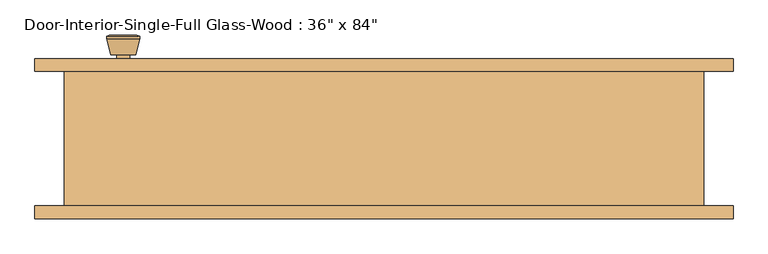
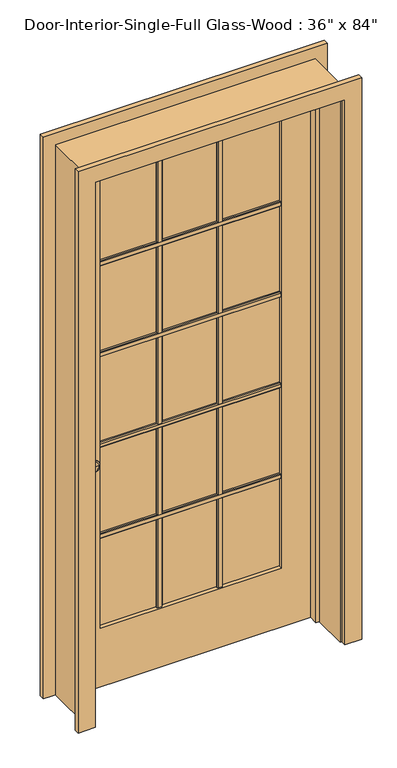
"""IFC4 building model written with IfcOpenShell, lengths in millimetres: door geometry."""

from ifc_helpers import new_model, si_unit, point, frame, frame_2d, origin, place, context, project, spatial, polyline, circle_curve, trimmed, segment, composite_curve, outline, extrude, faceted_brep, source, transform, mapped, element, save
from ifc_brep_helpers import plane_surface, cylinder_surface, revolved_surface, advanced_brep


def door_cfd81529(model_context):
    return source(origin(), model_context, "Body", "SolidModel", [
        extrude(outline(polyline([(84.455, 1667.51), (90.805, 1667.51), (93.98, 1664.335), (93.98, 1651.635), (90.805, 1648.46), (84.455, 1648.46), (84.455, 1667.51)])), frame((-336.55, 0.0, 0.0), z_axis=(1.0, 0.0, 0.0), x_axis=(0.0, 1.0, 0.0)), (0.0, 0.0, 1.0), 673.1),
        extrude(outline(polyline([(84.455, 1310.9575), (90.805, 1310.9575), (93.98, 1307.7825), (93.98, 1295.0825), (90.805, 1291.9075), (84.455, 1291.9075), (84.455, 1310.9575)])), frame((-336.55, 0.0, 0.0), z_axis=(1.0, 0.0, 0.0), x_axis=(0.0, 1.0, 0.0)), (0.0, 0.0, 1.0), 673.1),
        extrude(outline(polyline([(84.455, 954.405), (90.805, 954.405), (93.98, 951.23), (93.98, 938.53), (90.805, 935.355), (84.455, 935.355), (84.455, 954.405)])), frame((-336.55, 0.0, 0.0), z_axis=(1.0, 0.0, 0.0), x_axis=(0.0, 1.0, 0.0)), (0.0, 0.0, 1.0), 673.1),
        extrude(outline(polyline([(84.455, 597.8525), (90.805, 597.8525), (93.98, 594.6775), (93.98, 581.9775), (90.805, 578.8025), (84.455, 578.8025), (84.455, 597.8525)])), frame((-336.55, 0.0, 0.0), z_axis=(1.0, 0.0, 0.0), x_axis=(0.0, 1.0, 0.0)), (0.0, 0.0, 1.0), 673.1),
        extrude(outline(polyline([(102.6583333, 84.455), (102.6583333, 90.805), (105.8333333, 93.98), (118.5333333, 93.98), (121.7083333, 90.805), (121.7083333, 84.455), (102.6583333, 84.455)])), frame((0.0, 0.0, 231.775), z_axis=(0.0, 0.0, 1.0), x_axis=(1.0, 0.0, 0.0)), (0.0, 0.0, 1.0), 1782.7625),
        extrude(outline(polyline([(-121.7083333, 84.455), (-121.7083333, 90.805), (-118.5333333, 93.98), (-105.8333333, 93.98), (-102.6583333, 90.805), (-102.6583333, 84.455), (-121.7083333, 84.455)])), frame((0.0, 0.0, 231.775), z_axis=(0.0, 0.0, 1.0), x_axis=(1.0, 0.0, 0.0)), (0.0, 0.0, 1.0), 1782.7625),
        extrude(outline(polyline([(77.47, 1667.51), (77.47, 1648.46), (71.12, 1648.46), (67.945, 1651.635), (67.945, 1664.335), (71.12, 1667.51), (77.47, 1667.51)])), frame((-336.55, 0.0, 0.0), z_axis=(1.0, 0.0, 0.0), x_axis=(0.0, 1.0, 0.0)), (0.0, 0.0, 1.0), 673.1),
        extrude(outline(polyline([(77.47, 1310.9575), (77.47, 1291.9075), (71.12, 1291.9075), (67.945, 1295.0825), (67.945, 1307.7825), (71.12, 1310.9575), (77.47, 1310.9575)])), frame((-336.55, 0.0, 0.0), z_axis=(1.0, 0.0, 0.0), x_axis=(0.0, 1.0, 0.0)), (0.0, 0.0, 1.0), 673.1),
        extrude(outline(polyline([(77.47, 954.405), (77.47, 935.355), (71.12, 935.355), (67.945, 938.53), (67.945, 951.23), (71.12, 954.405), (77.47, 954.405)])), frame((-336.55, 0.0, 0.0), z_axis=(1.0, 0.0, 0.0), x_axis=(0.0, 1.0, 0.0)), (0.0, 0.0, 1.0), 673.1),
        extrude(outline(polyline([(77.47, 597.8525), (77.47, 578.8025), (71.12, 578.8025), (67.945, 581.9775), (67.945, 594.6775), (71.12, 597.8525), (77.47, 597.8525)])), frame((-336.55, 0.0, 0.0), z_axis=(1.0, 0.0, 0.0), x_axis=(0.0, 1.0, 0.0)), (0.0, 0.0, 1.0), 673.1),
        extrude(outline(polyline([(102.6583333, 77.47), (121.7083333, 77.47), (121.7083333, 71.12), (118.5333333, 67.945), (105.8333333, 67.945), (102.6583333, 71.12), (102.6583333, 77.47)])), frame((0.0, 0.0, 231.775), z_axis=(0.0, 0.0, 1.0), x_axis=(1.0, 0.0, 0.0)), (0.0, 0.0, 1.0), 1782.7625),
        extrude(outline(polyline([(-121.7083333, 77.47), (-102.6583333, 77.47), (-102.6583333, 71.12), (-105.8333333, 67.945), (-118.5333333, 67.945), (-121.7083333, 71.12), (-121.7083333, 77.47)])), frame((0.0, 0.0, 231.775), z_axis=(0.0, 0.0, 1.0), x_axis=(1.0, 0.0, 0.0)), (0.0, 0.0, 1.0), 1782.7625),
        advanced_brep(
        [(-393.7, 57.5, 914.4), (-383.7, 57.5, 914.4), (-403.7, 57.5, 914.4), (-373.2241324, 8.5, 914.4), (-393.7, 8.5, 914.4), (-414.1758676, 8.5, 914.4), (-368.7, 10.3278681, 914.4), (-418.7, 10.3278681, 914.4), (-368.7, 13.7915463, 914.4), (-418.7, 13.7915463, 914.4), (-375.063764, 38.5, 914.4), (-412.336236, 38.5, 914.4), (-383.7, 38.5, 914.4), (-403.7, 38.5, 914.4)],
        [
            (0, 1),
            (1, 2, circle_curve(frame((-393.7, 57.5, 914.4), z_axis=(0.0, 1.0, 0.0), x_axis=(-1.0, 0.0, 0.0)), 10.0)),
            (2, 0),
            (2, 1, circle_curve(frame((-393.7, 57.5, 914.4), z_axis=(0.0, 1.0, 0.0), x_axis=(-1.0, 0.0, 0.0)), 10.0)),
            (3, 4),
            (4, 5),
            (5, 3, circle_curve(frame((-393.7, 8.5, 914.4), z_axis=(0.0, -1.0, 0.0), x_axis=(-1.0, 0.0, 0.0)), 20.4758676)),
            (3, 5, circle_curve(frame((-393.7, 8.5, 914.4), z_axis=(0.0, -1.0, 0.0), x_axis=(-1.0, 0.0, 0.0)), 20.4758676)),
            (6, 3),
            (5, 7),
            (7, 6, circle_curve(frame((-393.7, 10.3278681, 914.4), z_axis=(0.0, -1.0, 0.0), x_axis=(-1.0, 0.0, 0.0)), 25.0)),
            (6, 7, circle_curve(frame((-393.7, 10.3278681, 914.4), z_axis=(0.0, -1.0, 0.0), x_axis=(-1.0, 0.0, 0.0)), 25.0)),
            (8, 6),
            (7, 9),
            (9, 8, circle_curve(frame((-393.7, 13.7915463, 914.4), z_axis=(0.0, -1.0, 0.0), x_axis=(-1.0, 0.0, 0.0)), 25.0)),
            (8, 9, circle_curve(frame((-393.7, 13.7915463, 914.4), z_axis=(0.0, -1.0, 0.0), x_axis=(-1.0, 0.0, 0.0)), 25.0)),
            (10, 8),
            (9, 11),
            (11, 10, circle_curve(frame((-393.7, 38.5, 914.4), z_axis=(0.0, -1.0, 0.0), x_axis=(-1.0, 0.0, 0.0)), 18.636236)),
            (10, 11, circle_curve(frame((-393.7, 38.5, 914.4), z_axis=(0.0, -1.0, 0.0), x_axis=(-1.0, 0.0, 0.0)), 18.636236)),
            (12, 10),
            (11, 13),
            (13, 12, circle_curve(frame((-393.7, 38.5, 914.4), z_axis=(0.0, -1.0, 0.0), x_axis=(-1.0, 0.0, 0.0)), 10.0)),
            (12, 13, circle_curve(frame((-393.7, 38.5, 914.4), z_axis=(0.0, -1.0, 0.0), x_axis=(-1.0, 0.0, 0.0)), 10.0)),
            (1, 12),
            (13, 2),
        ],
        [
            plane_surface(frame((-393.7, 57.5, 914.4), z_axis=(0.0, 1.0, 0.0), x_axis=(-1.0, 0.0, 0.0))),
            plane_surface(frame((-393.7, 8.5, 914.4), z_axis=(0.0, -1.0, 0.0), x_axis=(-1.0, 0.0, 0.0))),
            revolved_surface(polyline([(-414.1758676, 8.5, 914.4), (-418.7, 10.3278681, 914.4)]), (-393.7, 57.5, 914.4), (0.0, 1.0, 0.0)),
            cylinder_surface(frame((-393.7, 57.5, 914.4), z_axis=(0.0, 1.0, 0.0), x_axis=(-1.0, 0.0, 0.0)), 25.0),
            revolved_surface(polyline([(-418.7, 13.7915463, 914.4), (-412.336236, 38.5, 914.4)]), (-393.7, 57.5, 914.4), (0.0, 1.0, 0.0)),
            plane_surface(frame((-393.7, 38.5, 914.4), z_axis=(0.0, 1.0, 0.0), x_axis=(-1.0, 0.0, 0.0))),
            cylinder_surface(frame((-393.7, 57.5, 914.4), z_axis=(0.0, 1.0, 0.0), x_axis=(-1.0, 0.0, 0.0)), 10.0),
        ],
        [
            (0, [[1, 2, 3]]),
            (0, [[-3, 4, -1]]),
            (1, [[5, 6, 7]]),
            (1, [[-6, -5, 8]]),
            (2, [[9, -7, 10, 11]]),
            (2, [[-10, -8, -9, 12]]),
            (3, [[13, -11, 14, 15]]),
            (3, [[-14, -12, -13, 16]]),
            (4, [[17, -15, 18, 19]]),
            (4, [[-18, -16, -17, 20]]),
            (5, [[21, -19, 22, 23]]),
            (5, [[-22, -20, -21, 24]]),
            (6, [[25, -23, 26, -2]]),
            (6, [[-26, -24, -25, -4]]),
        ],
    ),
        extrude(outline(composite_curve([segment(trimmed(circle_curve(frame_2d((914.4, -393.7)), 30.0), [point((914.4, -423.7))], [point((914.4, -363.7))], False, "CARTESIAN"), True, "CONTINUOUS"), segment(trimmed(circle_curve(frame_2d((914.4, -393.7)), 30.0), [point((914.4, -363.7))], [point((914.4, -423.7))], False, "CARTESIAN"), True, "CONTINUOUS")], self_intersect=False)), frame((0.0, 57.5, 0.0), z_axis=(0.0, 1.0, 0.0), x_axis=(0.0, 0.0, 1.0)), (0.0, 0.0, 1.0), 6.0),
        advanced_brep(
        [(-393.7, 104.425, 914.4), (-403.7, 104.425, 914.4), (-383.7, 104.425, 914.4), (-373.2241324, 153.425, 914.4), (-414.1758676, 153.425, 914.4), (-393.7, 153.425, 914.4), (-368.7, 151.5971319, 914.4), (-418.7, 151.5971319, 914.4), (-368.7, 148.1334537, 914.4), (-418.7, 148.1334537, 914.4), (-375.063764, 123.425, 914.4), (-412.336236, 123.425, 914.4), (-383.7, 123.425, 914.4), (-403.7, 123.425, 914.4)],
        [
            (0, 1),
            (1, 2, circle_curve(frame((-393.7, 104.425, 914.4), z_axis=(0.0, -1.0, 0.0), x_axis=(-1.0, 0.0, 0.0)), 10.0)),
            (2, 0),
            (2, 1, circle_curve(frame((-393.7, 104.425, 914.4), z_axis=(0.0, -1.0, 0.0), x_axis=(-1.0, 0.0, 0.0)), 10.0)),
            (3, 4, circle_curve(frame((-393.7, 153.425, 914.4), z_axis=(0.0, 1.0, 0.0), x_axis=(-1.0, 0.0, 0.0)), 20.4758676)),
            (4, 5),
            (5, 3),
            (4, 3, circle_curve(frame((-393.7, 153.425, 914.4), z_axis=(0.0, 1.0, 0.0), x_axis=(-1.0, 0.0, 0.0)), 20.4758676)),
            (6, 7, circle_curve(frame((-393.7, 151.5971319, 914.4), z_axis=(0.0, 1.0, 0.0), x_axis=(-1.0, 0.0, 0.0)), 25.0)),
            (7, 4),
            (3, 6),
            (7, 6, circle_curve(frame((-393.7, 151.5971319, 914.4), z_axis=(0.0, 1.0, 0.0), x_axis=(-1.0, 0.0, 0.0)), 25.0)),
            (8, 9, circle_curve(frame((-393.7, 148.1334537, 914.4), z_axis=(0.0, 1.0, 0.0), x_axis=(-1.0, 0.0, 0.0)), 25.0)),
            (9, 7),
            (6, 8),
            (9, 8, circle_curve(frame((-393.7, 148.1334537, 914.4), z_axis=(0.0, 1.0, 0.0), x_axis=(-1.0, 0.0, 0.0)), 25.0)),
            (10, 11, circle_curve(frame((-393.7, 123.425, 914.4), z_axis=(0.0, 1.0, 0.0), x_axis=(-1.0, 0.0, 0.0)), 18.636236)),
            (11, 9),
            (8, 10),
            (11, 10, circle_curve(frame((-393.7, 123.425, 914.4), z_axis=(0.0, 1.0, 0.0), x_axis=(-1.0, 0.0, 0.0)), 18.636236)),
            (12, 13, circle_curve(frame((-393.7, 123.425, 914.4), z_axis=(0.0, 1.0, 0.0), x_axis=(-1.0, 0.0, 0.0)), 10.0)),
            (13, 11),
            (10, 12),
            (13, 12, circle_curve(frame((-393.7, 123.425, 914.4), z_axis=(0.0, 1.0, 0.0), x_axis=(-1.0, 0.0, 0.0)), 10.0)),
            (1, 13),
            (12, 2),
        ],
        [
            plane_surface(frame((-393.7, 104.425, 914.4), z_axis=(0.0, -1.0, 0.0), x_axis=(-1.0, 0.0, 0.0))),
            plane_surface(frame((-393.7, 153.425, 914.4), z_axis=(0.0, 1.0, 0.0), x_axis=(-1.0, 0.0, 0.0))),
            revolved_surface(polyline([(-414.1758676, 153.425, 914.4), (-418.7, 151.5971319, 914.4)]), (-393.7, 104.425, 914.4), (0.0, -1.0, 0.0)),
            cylinder_surface(frame((-393.7, 104.425, 914.4), z_axis=(0.0, -1.0, 0.0), x_axis=(-1.0, 0.0, 0.0)), 25.0),
            revolved_surface(polyline([(-418.7, 148.1334537, 914.4), (-412.336236, 123.425, 914.4)]), (-393.7, 104.425, 914.4), (0.0, -1.0, 0.0)),
            plane_surface(frame((-393.7, 123.425, 914.4), z_axis=(0.0, -1.0, 0.0), x_axis=(-1.0, 0.0, 0.0))),
            cylinder_surface(frame((-393.7, 104.425, 914.4), z_axis=(0.0, -1.0, 0.0), x_axis=(-1.0, 0.0, 0.0)), 10.0),
        ],
        [
            (0, [[1, 2, 3]]),
            (0, [[-3, 4, -1]]),
            (1, [[5, 6, 7]]),
            (1, [[8, -7, -6]]),
            (2, [[9, 10, -5, 11]]),
            (2, [[12, -11, -8, -10]]),
            (3, [[13, 14, -9, 15]]),
            (3, [[16, -15, -12, -14]]),
            (4, [[17, 18, -13, 19]]),
            (4, [[20, -19, -16, -18]]),
            (5, [[21, 22, -17, 23]]),
            (5, [[24, -23, -20, -22]]),
            (6, [[-2, 25, -21, 26]]),
            (6, [[-4, -26, -24, -25]]),
        ],
    ),
        extrude(outline(composite_curve([segment(trimmed(circle_curve(frame_2d((914.4, -393.7)), 30.0), [point((914.4, -423.7))], [point((914.4, -363.7))], False, "CARTESIAN"), True, "CONTINUOUS"), segment(trimmed(circle_curve(frame_2d((914.4, -393.7)), 30.0), [point((914.4, -363.7))], [point((914.4, -423.7))], False, "CARTESIAN"), True, "CONTINUOUS")], self_intersect=False)), frame((0.0, 98.425, 0.0), z_axis=(0.0, 1.0, 0.0), x_axis=(0.0, 0.0, 1.0)), (0.0, 0.0, 1.0), 6.0),
        extrude(outline(polyline([(2133.6, -457.2), (0.0, -457.2), (0.0, 457.2), (2133.6, 457.2), (2133.6, -457.2)]), holes=[polyline([(2014.5375, -336.55), (2014.5375, 336.55), (231.775, 336.55), (231.775, -336.55), (2014.5375, -336.55)])]), frame((0.0, 63.5, 0.0), z_axis=(0.0, 1.0, 0.0), x_axis=(0.0, 0.0, 1.0)), (0.0, 0.0, 1.0), 34.925),
        faceted_brep([(482.6, 98.425, 0.0), (482.6, -104.775, 0.0), (457.2, -104.775, 0.0), (457.2, 28.575, 0.0), (444.5, 28.575, 0.0), (444.5, 63.5, 0.0), (457.2, 63.5, 0.0), (457.2, 98.425, 0.0), (482.6, 98.425, 2159.0), (482.6, -104.775, 2159.0), (-482.6, -104.775, 2159.0), (-482.6, -104.775, 0.0), (-457.2, -104.775, 0.0), (-457.2, -104.775, 2133.6), (457.2, -104.775, 2133.6), (457.2, 28.575, 2133.6), (-457.2, 28.575, 2133.6), (-457.2, 28.575, 0.0), (-444.5, 28.575, 0.0), (-444.5, 28.575, 2120.9), (444.5, 28.575, 2120.9), (444.5, 63.5, 2120.9), (-444.5, 63.5, 2120.9), (-444.5, 63.5, 0.0), (-457.2, 63.5, 0.0), (-457.2, 63.5, 2133.6), (457.2, 63.5, 2133.6), (457.2, 98.425, 2133.6), (-457.2, 98.425, 2133.6), (-457.2, 98.425, 0.0), (-482.6, 98.425, 0.0), (-482.6, 98.425, 2159.0)], [[[0, 1, 2, 3, 4, 5, 6, 7]], [[1, 0, 8, 9]], [[2, 1, 9, 10, 11, 12, 13, 14]], [[3, 2, 14, 15]], [[4, 3, 15, 16, 17, 18, 19, 20]], [[5, 4, 20, 21]], [[6, 5, 21, 22, 23, 24, 25, 26]], [[7, 6, 26, 27]], [[0, 7, 27, 28, 29, 30, 31, 8]], [[9, 8, 31, 10]], [[15, 14, 13, 16]], [[21, 20, 19, 22]], [[27, 26, 25, 28]], [[30, 29, 24, 23, 18, 17, 12, 11]], [[10, 31, 30, 11]], [[16, 13, 12, 17]], [[22, 19, 18, 23]], [[28, 25, 24, 29]]]),
        extrude(outline(polyline([(336.55, 77.47), (-336.55, 77.47), (-336.55, 84.455), (336.55, 84.455), (336.55, 77.47)])), frame((0.0, 0.0, 231.775), z_axis=(0.0, 0.0, 1.0), x_axis=(1.0, 0.0, 0.0)), (0.0, 0.0, 1.0), 1782.7625),
        extrude(outline(polyline([(0.0, 463.55), (0.0, 527.05), (2203.45, 527.05), (2203.45, -527.05), (0.0, -527.05), (0.0, -463.55), (2139.95, -463.55), (2139.95, 463.55), (0.0, 463.55)])), frame((0.0, -123.825, 0.0), z_axis=(0.0, 1.0, 0.0), x_axis=(0.0, 0.0, 1.0)), (0.0, 0.0, 1.0), 19.05),
        extrude(outline(polyline([(0.0, 463.55), (0.0, 527.05), (2203.45, 527.05), (2203.45, -527.05), (0.0, -527.05), (0.0, -463.55), (2139.95, -463.55), (2139.95, 463.55), (0.0, 463.55)])), frame((0.0, 98.425, 0.0), z_axis=(0.0, 1.0, 0.0), x_axis=(0.0, 0.0, 1.0)), (0.0, 0.0, 1.0), 19.05),
    ])


if __name__ == "__main__":
    model = new_model("IFC4")
    model_context = context("Model", 3, world=origin())
    ifc_project = project(units=[si_unit("LENGTHUNIT", "METRE", prefix="MILLI")], contexts=[model_context])
    site = spatial("IfcSite", under=ifc_project)
    building = spatial("IfcBuilding", under=site)
    placement = place(None, origin())
    door_shape = door_cfd81529(model_context)
    element("IfcDoor", 1, ObjectType="Door-Interior-Single-Full Glass-Wood : 36\" x 84\"", at=placement, inside=building, context=model_context, shape_type="MappedRepresentation", body=[
        mapped(door_shape, transform((0.0, 0.0, 0.0), x_axis=(1.0, 0.0, 0.0), y_axis=(0.0, 1.0, 0.0), z_axis=(0.0, 0.0, 1.0))),
    ])
    save(model, "model.ifc")

# Revit data of these elements
# Type "Door-Interior-Single-Full Glass-Wood : 36\" x 84\""
#   Type Mark = "11"
#   Assembly Code = "C1020300"
#   Analytic Construction = "Wood frame with single clear glass"
#   Top Rail = 0' - 4 11/16"
#   Thickness = 0' - 1 3/8"
#   Thermal Resistance (R) = 1.0102 (h·ft²·°F)/BTU
#   Swing Angle [instance default] = 90.00°
#   Stiles = 0' - 4 3/4"
#   Rough Width = 3' - 2"
#   Rough Height = 7' - 1"
#   Height = 7' - 0"
#   Width = 3' - 0"
#   Heat Transfer Coefficient (U) = 0.9900 BTU/(h·ft²·°F)
#   Bottom Rail = 0' - 9 1/8"
#   Show Grill [instance default] = yes
#   Trim Material = Cherry
#   Panel Material = Cherry
#   Frame Material = Cherry
#   Door Handle Material = Aluminum
#   Visual Light Transmittance = 0
#   Solar Heat Gain Coefficient = 0
#   Wall Closure = (empty or 0)
#   Function = (empty or 0)
# Element 1 (IfcDoor, "Door-Interior-Single-Full Glass-Wood : 36\" x 84\"")
#   Materials on its faces: "Cherry", "Aluminum", "Glass"
# Materials
#   "Cherry": class "Wood", colour RGB 226 177 128, transparency 0, Description = "Prunus Serotina", Cost = 0
#   "Aluminum": class "Metal", colour RGB 247 247 247, transparency 0, Description = "Aluminum 6061", Cost = 0
#   "Glass": class "Glass", colour RGB 0 128 192, transparency 0.75, Description = "Soda Lime Glass", Cost = 0
